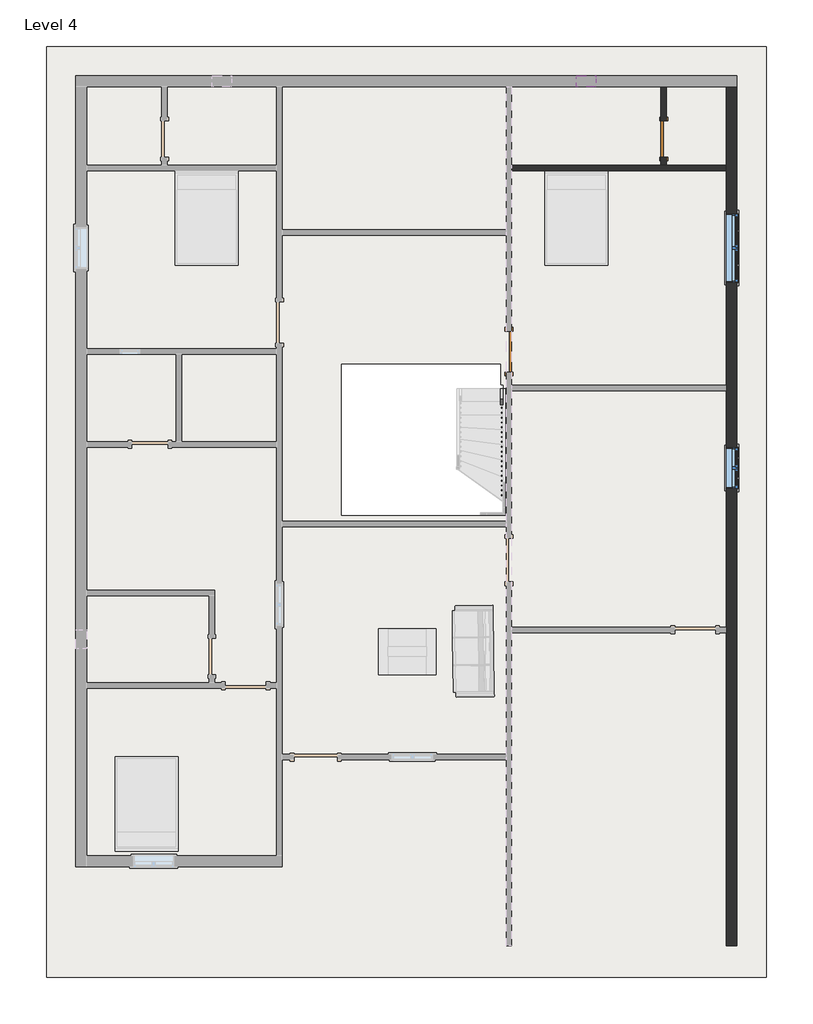
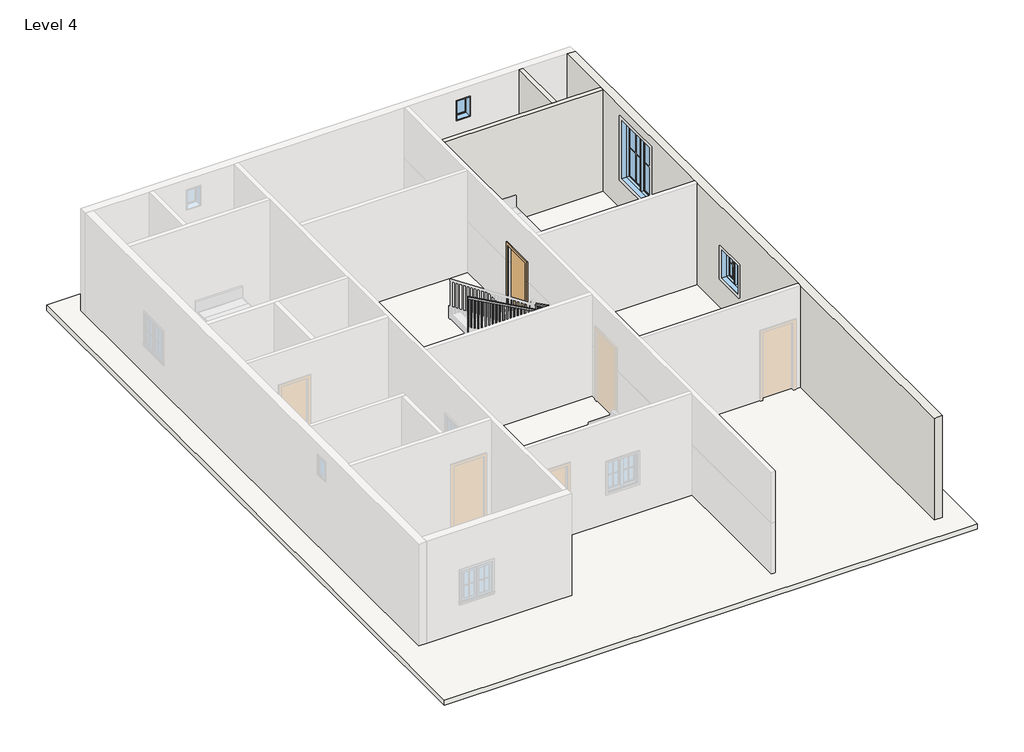
# One storey, part 2 of 3: 3 walls, 3 windows, 2 doors, 1 railing, 1 roof.
"""IFC4 building model written with IfcOpenShell, lengths in millimetres."""

from ifc_helpers import new_model, si_unit, frame, origin, place, context, project, spatial, polyline, outline, extrude, faceted_brep, transform, mapped, element, save
from components import door_f2b275c1, door_c29894e6, window_aa618e30, window_339605e1, window_9ac97e1a

model = new_model("IFC4")

# Units and contexts
model_context = context("Model", 3, world=origin())
ifc_project = project(units=[si_unit("LENGTHUNIT", "METRE", prefix="MILLI")], contexts=[model_context])

# Site, building, storey
site = spatial("IfcSite", under=ifc_project)
building = spatial("IfcBuilding", under=site)
storey = spatial("IfcBuildingStorey", under=building, Name="Level 4", Elevation=6400.8)

# Doors
placement = place(None, origin())
door_shape = door_f2b275c1(model_context)
element("IfcDoor", 1, ObjectType="Single-Flush : 30\" x 80\"", at=placement, inside=storey, context=model_context, shape_type="MappedRepresentation", body=[
    mapped(door_shape, transform((4827.3366507, 9100.7522623, 6400.8), x_axis=(0.0, -1.0, 0.0), y_axis=(1.0, 0.0, 0.0), z_axis=(0.0, 0.0, 1.0))),
])
door_2_shape = door_c29894e6(model_context)
element("IfcDoor", 2, ObjectType="Single-Flush : 34\" x 80\"", at=placement, inside=storey, context=model_context, shape_type="MappedRepresentation", body=[
    mapped(door_2_shape, transform((1583.2084916, 4643.0522623, 6400.8), x_axis=(0.0, -1.0, 0.0), y_axis=(1.0, 0.0, 0.0), z_axis=(0.0, 0.0, 1.0))),
])

# Railing
element("IfcRailing", 3, ObjectType="Handrail - Rectangular", at=placement, inside=storey, context=model_context, shape_type="SolidModel", body=[
    faceted_brep([(1456.2084916, 3870.4222402, 7484.5333333), (1456.2084916, 3870.4222402, 7427.5391458), (1405.4084916, 3870.4222402, 7427.5391458), (1405.4084916, 3870.4222402, 7484.5333333), (1456.2084916, 1506.6647172, 8686.878212), (1456.2084916, 1494.487215, 8636.078212), (1405.4084916, 1494.487215, 8636.078212), (1405.4084916, 1506.6647172, 8686.878212), (1456.2084916, 1268.9652728, 8686.878212), (1456.2084916, 1268.9652728, 8636.078212), (1405.4084916, 1319.7652728, 8636.078212), (1405.4084916, 1319.7652728, 8686.878212), (1234.4478889, 1268.9652728, 8686.878212), (1221.4006723, 1268.9652728, 8636.078212), (1221.4006723, 1319.7652728, 8636.078212), (1234.4478889, 1319.7652728, 8686.878212), (-1813.7050583, 1268.9652728, 10363.2), (-1813.7050583, 1319.7652728, 10363.2), (-1813.7050583, 1319.7652728, 10305.2247257), (-1813.7050583, 1268.9652728, 10305.2247257)], [[[0, 1, 2, 3]], [[1, 0, 4, 5]], [[2, 1, 5, 6]], [[3, 2, 6, 7]], [[0, 3, 7, 4]], [[5, 4, 8, 9]], [[6, 5, 9, 10]], [[7, 6, 10, 11]], [[4, 7, 11, 8]], [[9, 8, 12, 13]], [[10, 9, 13, 14]], [[11, 10, 14, 15]], [[8, 11, 15, 12]], [[16, 17, 18, 19]], [[13, 12, 16, 19]], [[14, 13, 19, 18]], [[15, 14, 18, 17]], [[12, 15, 17, 16]]]),
    extrude(outline(polyline([(10258.2655707, -1728.3165084), (9279.4666667, -1728.3165084), (9279.4666667, -1709.2665084), (10247.7890853, -1709.2665084), (10258.2655707, -1728.3165084)])), frame((0.0, 1284.8402728, 0.0), z_axis=(0.0, 1.0, 0.0), x_axis=(0.0, 0.0, 1.0)), (0.0, 0.0, 1.0), 19.05),
    extrude(outline(polyline([(10202.3909816, -1626.7165084), (9279.4666667, -1626.7165084), (9279.4666667, -1607.6665084), (10191.9144961, -1607.6665084), (10202.3909816, -1626.7165084)])), frame((0.0, 1284.8402728, 0.0), z_axis=(0.0, 1.0, 0.0), x_axis=(0.0, 0.0, 1.0)), (0.0, 0.0, 1.0), 19.05),
    extrude(outline(polyline([(10146.5163924, -1525.1165084), (9110.1333333, -1525.1165084), (9110.1333333, -1506.0665084), (10136.0399069, -1506.0665084), (10146.5163924, -1525.1165084)])), frame((0.0, 1284.8402728, 0.0), z_axis=(0.0, 1.0, 0.0), x_axis=(0.0, 0.0, 1.0)), (0.0, 0.0, 1.0), 19.05),
    extrude(outline(polyline([(10090.6418032, -1423.5165084), (9110.1333333, -1423.5165084), (9110.1333333, -1404.4665084), (10080.1653177, -1404.4665084), (10090.6418032, -1423.5165084)])), frame((0.0, 1284.8402728, 0.0), z_axis=(0.0, 1.0, 0.0), x_axis=(0.0, 0.0, 1.0)), (0.0, 0.0, 1.0), 19.05),
    extrude(outline(polyline([(10034.767214, -1321.9165084), (9110.1333333, -1321.9165084), (9110.1333333, -1302.8665084), (10024.2907286, -1302.8665084), (10034.767214, -1321.9165084)])), frame((0.0, 1284.8402728, 0.0), z_axis=(0.0, 1.0, 0.0), x_axis=(0.0, 0.0, 1.0)), (0.0, 0.0, 1.0), 19.05),
    extrude(outline(polyline([(9978.8926249, -1220.3165084), (8940.8, -1220.3165084), (8940.8, -1201.2665084), (9968.4161394, -1201.2665084), (9978.8926249, -1220.3165084)])), frame((0.0, 1284.8402728, 0.0), z_axis=(0.0, 1.0, 0.0), x_axis=(0.0, 0.0, 1.0)), (0.0, 0.0, 1.0), 19.05),
    extrude(outline(polyline([(9923.0180357, -1118.7165084), (8940.8, -1118.7165084), (8940.8, -1099.6665084), (9912.5415502, -1099.6665084), (9923.0180357, -1118.7165084)])), frame((0.0, 1284.8402728, 0.0), z_axis=(0.0, 1.0, 0.0), x_axis=(0.0, 0.0, 1.0)), (0.0, 0.0, 1.0), 19.05),
    extrude(outline(polyline([(9867.1434465, -1017.1165084), (8940.8, -1017.1165084), (8940.8, -998.0665084), (9856.666961, -998.0665084), (9867.1434465, -1017.1165084)])), frame((0.0, 1284.8402728, 0.0), z_axis=(0.0, 1.0, 0.0), x_axis=(0.0, 0.0, 1.0)), (0.0, 0.0, 1.0), 19.05),
    extrude(outline(polyline([(9811.2688573, -915.5165084), (8771.4666667, -915.5165084), (8771.4666667, -896.4665084), (9800.7923719, -896.4665084), (9811.2688573, -915.5165084)])), frame((0.0, 1284.8402728, 0.0), z_axis=(0.0, 1.0, 0.0), x_axis=(0.0, 0.0, 1.0)), (0.0, 0.0, 1.0), 19.05),
    extrude(outline(polyline([(9755.3942682, -813.9165084), (8771.4666667, -813.9165084), (8771.4666667, -794.8665084), (9744.9177827, -794.8665084), (9755.3942682, -813.9165084)])), frame((0.0, 1284.8402728, 0.0), z_axis=(0.0, 1.0, 0.0), x_axis=(0.0, 0.0, 1.0)), (0.0, 0.0, 1.0), 19.05),
    extrude(outline(polyline([(9699.519679, -712.3165084), (8771.4666667, -712.3165084), (8771.4666667, -693.2665084), (9689.0431935, -693.2665084), (9699.519679, -712.3165084)])), frame((0.0, 1284.8402728, 0.0), z_axis=(0.0, 1.0, 0.0), x_axis=(0.0, 0.0, 1.0)), (0.0, 0.0, 1.0), 19.05),
    extrude(outline(polyline([(9643.6450898, -610.7165084), (8602.1333333, -610.7165084), (8602.1333333, -591.6665084), (9633.1686044, -591.6665084), (9643.6450898, -610.7165084)])), frame((0.0, 1284.8402728, 0.0), z_axis=(0.0, 1.0, 0.0), x_axis=(0.0, 0.0, 1.0)), (0.0, 0.0, 1.0), 19.05),
    extrude(outline(polyline([(9587.7705007, -509.1165084), (8602.1333333, -509.1165084), (8602.1333333, -490.0665084), (9577.2940152, -490.0665084), (9587.7705007, -509.1165084)])), frame((0.0, 1284.8402728, 0.0), z_axis=(0.0, 1.0, 0.0), x_axis=(0.0, 0.0, 1.0)), (0.0, 0.0, 1.0), 19.05),
    extrude(outline(polyline([(9531.8959115, -407.5165084), (8602.1333333, -407.5165084), (8602.1333333, -388.4665084), (9521.419426, -388.4665084), (9531.8959115, -407.5165084)])), frame((0.0, 1284.8402728, 0.0), z_axis=(0.0, 1.0, 0.0), x_axis=(0.0, 0.0, 1.0)), (0.0, 0.0, 1.0), 19.05),
    extrude(outline(polyline([(9476.0213223, -305.9165084), (8432.8, -305.9165084), (8432.8, -286.8665084), (9465.5448368, -286.8665084), (9476.0213223, -305.9165084)])), frame((0.0, 1284.8402728, 0.0), z_axis=(0.0, 1.0, 0.0), x_axis=(0.0, 0.0, 1.0)), (0.0, 0.0, 1.0), 19.05),
    extrude(outline(polyline([(9420.1467331, -204.3165084), (8432.8, -204.3165084), (8432.8, -185.2665084), (9409.6702477, -185.2665084), (9420.1467331, -204.3165084)])), frame((0.0, 1284.8402728, 0.0), z_axis=(0.0, 1.0, 0.0), x_axis=(0.0, 0.0, 1.0)), (0.0, 0.0, 1.0), 19.05),
    extrude(outline(polyline([(9364.272144, -102.7165084), (8432.8, -102.7165084), (8432.8, -83.6665084), (9353.7956585, -83.6665084), (9364.272144, -102.7165084)])), frame((0.0, 1284.8402728, 0.0), z_axis=(0.0, 1.0, 0.0), x_axis=(0.0, 0.0, 1.0)), (0.0, 0.0, 1.0), 19.05),
    extrude(outline(polyline([(9308.3975548, -1.1165084), (8263.4666667, -1.1165084), (8263.4666667, 17.9334916), (9297.9210693, 17.9334916), (9308.3975548, -1.1165084)])), frame((0.0, 1284.8402728, 0.0), z_axis=(0.0, 1.0, 0.0), x_axis=(0.0, 0.0, 1.0)), (0.0, 0.0, 1.0), 19.05),
    extrude(outline(polyline([(9252.5229656, 100.4834916), (8263.4666667, 100.4834916), (8263.4666667, 119.5334916), (9242.0464801, 119.5334916), (9252.5229656, 100.4834916)])), frame((0.0, 1284.8402728, 0.0), z_axis=(0.0, 1.0, 0.0), x_axis=(0.0, 0.0, 1.0)), (0.0, 0.0, 1.0), 19.05),
    extrude(outline(polyline([(9196.6483764, 202.0834916), (8263.4666667, 202.0834916), (8263.4666667, 221.1334916), (9186.171891, 221.1334916), (9196.6483764, 202.0834916)])), frame((0.0, 1284.8402728, 0.0), z_axis=(0.0, 1.0, 0.0), x_axis=(0.0, 0.0, 1.0)), (0.0, 0.0, 1.0), 19.05),
    extrude(outline(polyline([(9140.7737873, 303.6834916), (8094.1333333, 303.6834916), (8094.1333333, 322.7334916), (9130.2973018, 322.7334916), (9140.7737873, 303.6834916)])), frame((0.0, 1284.8402728, 0.0), z_axis=(0.0, 1.0, 0.0), x_axis=(0.0, 0.0, 1.0)), (0.0, 0.0, 1.0), 19.05),
    extrude(outline(polyline([(9084.8991981, 405.2834916), (8094.1333333, 405.2834916), (8094.1333333, 424.3334916), (9074.4227126, 424.3334916), (9084.8991981, 405.2834916)])), frame((0.0, 1284.8402728, 0.0), z_axis=(0.0, 1.0, 0.0), x_axis=(0.0, 0.0, 1.0)), (0.0, 0.0, 1.0), 19.05),
    extrude(outline(polyline([(9029.0246089, 506.8834916), (8094.1333333, 506.8834916), (8094.1333333, 525.9334916), (9018.5481235, 525.9334916), (9029.0246089, 506.8834916)])), frame((0.0, 1284.8402728, 0.0), z_axis=(0.0, 1.0, 0.0), x_axis=(0.0, 0.0, 1.0)), (0.0, 0.0, 1.0), 19.05),
    extrude(outline(polyline([(8973.1500198, 608.4834916), (7924.8, 608.4834916), (7924.8, 627.5334916), (8962.6735343, 627.5334916), (8973.1500198, 608.4834916)])), frame((0.0, 1284.8402728, 0.0), z_axis=(0.0, 1.0, 0.0), x_axis=(0.0, 0.0, 1.0)), (0.0, 0.0, 1.0), 19.05),
    extrude(outline(polyline([(8917.2754306, 710.0834916), (7924.8, 710.0834916), (7924.8, 729.1334916), (8906.7989451, 729.1334916), (8917.2754306, 710.0834916)])), frame((0.0, 1284.8402728, 0.0), z_axis=(0.0, 1.0, 0.0), x_axis=(0.0, 0.0, 1.0)), (0.0, 0.0, 1.0), 19.05),
    extrude(outline(polyline([(8861.4008414, 811.6834916), (7924.8, 811.6834916), (7924.8, 830.7334916), (8850.9243559, 830.7334916), (8861.4008414, 811.6834916)])), frame((0.0, 1284.8402728, 0.0), z_axis=(0.0, 1.0, 0.0), x_axis=(0.0, 0.0, 1.0)), (0.0, 0.0, 1.0), 19.05),
    extrude(outline(polyline([(8805.5262522, 913.2834916), (7924.8, 913.2834916), (7924.8, 932.3334916), (8795.0497668, 932.3334916), (8805.5262522, 913.2834916)])), frame((0.0, 1284.8402728, 0.0), z_axis=(0.0, 1.0, 0.0), x_axis=(0.0, 0.0, 1.0)), (0.0, 0.0, 1.0), 19.05),
    extrude(outline(polyline([(8749.6516631, 1014.8834916), (7755.4666667, 1014.8834916), (7755.4666667, 1033.9334916), (8739.1751776, 1033.9334916), (8749.6516631, 1014.8834916)])), frame((0.0, 1284.8402728, 0.0), z_axis=(0.0, 1.0, 0.0), x_axis=(0.0, 0.0, 1.0)), (0.0, 0.0, 1.0), 19.05),
    extrude(outline(polyline([(8693.7770739, 1116.4834916), (7755.4666667, 1116.4834916), (7755.4666667, 1135.5334916), (8683.3005884, 1135.5334916), (8693.7770739, 1116.4834916)])), frame((0.0, 1284.8402728, 0.0), z_axis=(0.0, 1.0, 0.0), x_axis=(0.0, 0.0, 1.0)), (0.0, 0.0, 1.0), 19.05),
    extrude(outline(polyline([(8637.9024847, 1218.0834916), (7755.4666667, 1218.0834916), (7755.4666667, 1237.1334916), (8627.4259992, 1237.1334916), (8637.9024847, 1218.0834916)])), frame((0.0, 1284.8402728, 0.0), z_axis=(0.0, 1.0, 0.0), x_axis=(0.0, 0.0, 1.0)), (0.0, 0.0, 1.0), 19.05),
    extrude(outline(polyline([(1338.7334916, 1284.8402728), (1319.6834916, 1284.8402728), (1319.6834916, 1303.8902728), (1338.7334916, 1303.8902728), (1338.7334916, 1284.8402728)])), frame((0.0, 0.0, 7755.4666667), z_axis=(0.0, 0.0, 1.0), x_axis=(1.0, 0.0, 0.0)), (0.0, 0.0, 1.0), 880.6115453),
    extrude(outline(polyline([(1440.3334916, 1339.9472402), (1440.3334916, 1320.8972402), (1421.2834916, 1320.8972402), (1421.2834916, 1339.9472402), (1440.3334916, 1339.9472402)])), frame((0.0, 0.0, 7755.4666667), z_axis=(0.0, 0.0, 1.0), x_axis=(1.0, 0.0, 0.0)), (0.0, 0.0, 1.0), 880.6115453),
    extrude(outline(polyline([(1440.3334916, 1441.5472402), (1440.3334916, 1422.4972402), (1421.2834916, 1422.4972402), (1421.2834916, 1441.5472402), (1440.3334916, 1441.5472402)])), frame((0.0, 0.0, 7755.4666667), z_axis=(0.0, 0.0, 1.0), x_axis=(1.0, 0.0, 0.0)), (0.0, 0.0, 1.0), 880.6115453),
    extrude(outline(polyline([(1543.1472402, 8611.3268864), (1543.1472402, 7755.4666667), (1524.0972402, 7755.4666667), (1524.0972402, 8621.016827), (1543.1472402, 8611.3268864)])), frame((1421.2834916, 0.0, 0.0), z_axis=(1.0, 0.0, 0.0), x_axis=(0.0, 1.0, 0.0)), (0.0, 0.0, 1.0), 19.05),
    extrude(outline(polyline([(1644.7472402, 8559.6472033), (1644.7472402, 7586.1333333), (1625.6972402, 7586.1333333), (1625.6972402, 8569.3371439), (1644.7472402, 8559.6472033)])), frame((1421.2834916, 0.0, 0.0), z_axis=(1.0, 0.0, 0.0), x_axis=(0.0, 1.0, 0.0)), (0.0, 0.0, 1.0), 19.05),
    extrude(outline(polyline([(1746.3472402, 8507.9675203), (1746.3472402, 7586.1333333), (1727.2972402, 7586.1333333), (1727.2972402, 8517.6574608), (1746.3472402, 8507.9675203)])), frame((1421.2834916, 0.0, 0.0), z_axis=(1.0, 0.0, 0.0), x_axis=(0.0, 1.0, 0.0)), (0.0, 0.0, 1.0), 19.05),
    extrude(outline(polyline([(1847.9472402, 8456.2878372), (1847.9472402, 7586.1333333), (1828.8972402, 7586.1333333), (1828.8972402, 8465.9777778), (1847.9472402, 8456.2878372)])), frame((1421.2834916, 0.0, 0.0), z_axis=(1.0, 0.0, 0.0), x_axis=(0.0, 1.0, 0.0)), (0.0, 0.0, 1.0), 19.05),
    extrude(outline(polyline([(1949.5472402, 8404.6081541), (1949.5472402, 7586.1333333), (1930.4972402, 7586.1333333), (1930.4972402, 8414.2980947), (1949.5472402, 8404.6081541)])), frame((1421.2834916, 0.0, 0.0), z_axis=(1.0, 0.0, 0.0), x_axis=(0.0, 1.0, 0.0)), (0.0, 0.0, 1.0), 19.05),
    extrude(outline(polyline([(2051.1472402, 8352.928471), (2051.1472402, 7416.8), (2032.0972402, 7416.8), (2032.0972402, 8362.6184116), (2051.1472402, 8352.928471)])), frame((1421.2834916, 0.0, 0.0), z_axis=(1.0, 0.0, 0.0), x_axis=(0.0, 1.0, 0.0)), (0.0, 0.0, 1.0), 19.05),
    extrude(outline(polyline([(2152.7472402, 8301.2487879), (2152.7472402, 7416.8), (2133.6972402, 7416.8), (2133.6972402, 8310.9387285), (2152.7472402, 8301.2487879)])), frame((1421.2834916, 0.0, 0.0), z_axis=(1.0, 0.0, 0.0), x_axis=(0.0, 1.0, 0.0)), (0.0, 0.0, 1.0), 19.05),
    extrude(outline(polyline([(2254.3472402, 8249.5691048), (2254.3472402, 7416.8), (2235.2972402, 7416.8), (2235.2972402, 8259.2590454), (2254.3472402, 8249.5691048)])), frame((1421.2834916, 0.0, 0.0), z_axis=(1.0, 0.0, 0.0), x_axis=(0.0, 1.0, 0.0)), (0.0, 0.0, 1.0), 19.05),
    extrude(outline(polyline([(2355.9472402, 8197.8894218), (2355.9472402, 7416.8), (2336.8972402, 7416.8), (2336.8972402, 8207.5793623), (2355.9472402, 8197.8894218)])), frame((1421.2834916, 0.0, 0.0), z_axis=(1.0, 0.0, 0.0), x_axis=(0.0, 1.0, 0.0)), (0.0, 0.0, 1.0), 19.05),
    extrude(outline(polyline([(2457.5472402, 8146.2097387), (2457.5472402, 7247.4666667), (2438.4972402, 7247.4666667), (2438.4972402, 8155.8996793), (2457.5472402, 8146.2097387)])), frame((1421.2834916, 0.0, 0.0), z_axis=(1.0, 0.0, 0.0), x_axis=(0.0, 1.0, 0.0)), (0.0, 0.0, 1.0), 19.05),
    extrude(outline(polyline([(2559.1472402, 8094.5300556), (2559.1472402, 7247.4666667), (2540.0972402, 7247.4666667), (2540.0972402, 8104.2199962), (2559.1472402, 8094.5300556)])), frame((1421.2834916, 0.0, 0.0), z_axis=(1.0, 0.0, 0.0), x_axis=(0.0, 1.0, 0.0)), (0.0, 0.0, 1.0), 19.05),
    extrude(outline(polyline([(2660.7472402, 8042.8503725), (2660.7472402, 7247.4666667), (2641.6972402, 7247.4666667), (2641.6972402, 8052.5403131), (2660.7472402, 8042.8503725)])), frame((1421.2834916, 0.0, 0.0), z_axis=(1.0, 0.0, 0.0), x_axis=(0.0, 1.0, 0.0)), (0.0, 0.0, 1.0), 19.05),
    extrude(outline(polyline([(2762.3472402, 7991.1706894), (2762.3472402, 7078.1333333), (2743.2972402, 7078.1333333), (2743.2972402, 8000.86063), (2762.3472402, 7991.1706894)])), frame((1421.2834916, 0.0, 0.0), z_axis=(1.0, 0.0, 0.0), x_axis=(0.0, 1.0, 0.0)), (0.0, 0.0, 1.0), 19.05),
    extrude(outline(polyline([(2863.9472402, 7939.4910064), (2863.9472402, 7078.1333333), (2844.8972402, 7078.1333333), (2844.8972402, 7949.1809469), (2863.9472402, 7939.4910064)])), frame((1421.2834916, 0.0, 0.0), z_axis=(1.0, 0.0, 0.0), x_axis=(0.0, 1.0, 0.0)), (0.0, 0.0, 1.0), 19.05),
    extrude(outline(polyline([(2965.5472402, 7887.8113233), (2965.5472402, 7078.1333333), (2946.4972402, 7078.1333333), (2946.4972402, 7897.5012638), (2965.5472402, 7887.8113233)])), frame((1421.2834916, 0.0, 0.0), z_axis=(1.0, 0.0, 0.0), x_axis=(0.0, 1.0, 0.0)), (0.0, 0.0, 1.0), 19.05),
    extrude(outline(polyline([(3067.1472402, 7836.1316402), (3067.1472402, 6908.8), (3048.0972402, 6908.8), (3048.0972402, 7845.8215808), (3067.1472402, 7836.1316402)])), frame((1421.2834916, 0.0, 0.0), z_axis=(1.0, 0.0, 0.0), x_axis=(0.0, 1.0, 0.0)), (0.0, 0.0, 1.0), 19.05),
    extrude(outline(polyline([(3168.7472402, 7784.4519571), (3168.7472402, 6908.8), (3149.6972402, 6908.8), (3149.6972402, 7794.1418977), (3168.7472402, 7784.4519571)])), frame((1421.2834916, 0.0, 0.0), z_axis=(1.0, 0.0, 0.0), x_axis=(0.0, 1.0, 0.0)), (0.0, 0.0, 1.0), 19.05),
    extrude(outline(polyline([(3270.3472402, 7732.772274), (3270.3472402, 6908.8), (3251.2972402, 6908.8), (3251.2972402, 7742.4622146), (3270.3472402, 7732.772274)])), frame((1421.2834916, 0.0, 0.0), z_axis=(1.0, 0.0, 0.0), x_axis=(0.0, 1.0, 0.0)), (0.0, 0.0, 1.0), 19.05),
    extrude(outline(polyline([(3371.9472402, 7681.0925909), (3371.9472402, 6739.4666667), (3352.8972402, 6739.4666667), (3352.8972402, 7690.7825315), (3371.9472402, 7681.0925909)])), frame((1421.2834916, 0.0, 0.0), z_axis=(1.0, 0.0, 0.0), x_axis=(0.0, 1.0, 0.0)), (0.0, 0.0, 1.0), 19.05),
    extrude(outline(polyline([(3473.5472402, 7629.4129079), (3473.5472402, 6739.4666667), (3454.4972402, 6739.4666667), (3454.4972402, 7639.1028484), (3473.5472402, 7629.4129079)])), frame((1421.2834916, 0.0, 0.0), z_axis=(1.0, 0.0, 0.0), x_axis=(0.0, 1.0, 0.0)), (0.0, 0.0, 1.0), 19.05),
    extrude(outline(polyline([(3575.1472402, 7577.7332248), (3575.1472402, 6739.4666667), (3556.0972402, 6739.4666667), (3556.0972402, 7587.4231654), (3575.1472402, 7577.7332248)])), frame((1421.2834916, 0.0, 0.0), z_axis=(1.0, 0.0, 0.0), x_axis=(0.0, 1.0, 0.0)), (0.0, 0.0, 1.0), 19.05),
    extrude(outline(polyline([(3676.7472402, 7526.0535417), (3676.7472402, 6570.1333333), (3657.6972402, 6570.1333333), (3657.6972402, 7535.7434823), (3676.7472402, 7526.0535417)])), frame((1421.2834916, 0.0, 0.0), z_axis=(1.0, 0.0, 0.0), x_axis=(0.0, 1.0, 0.0)), (0.0, 0.0, 1.0), 19.05),
    extrude(outline(polyline([(3778.3472402, 7474.3738586), (3778.3472402, 6570.1333333), (3759.2972402, 6570.1333333), (3759.2972402, 7484.0637992), (3778.3472402, 7474.3738586)])), frame((1421.2834916, 0.0, 0.0), z_axis=(1.0, 0.0, 0.0), x_axis=(0.0, 1.0, 0.0)), (0.0, 0.0, 1.0), 19.05),
    extrude(outline(polyline([(1440.3334916, 1303.8902728), (1440.3334916, 1284.8402728), (1421.2834916, 1284.8402728), (1421.2834916, 1303.8902728), (1440.3334916, 1303.8902728)])), frame((0.0, 0.0, 7755.4666667), z_axis=(0.0, 0.0, 1.0), x_axis=(1.0, 0.0, 0.0)), (0.0, 0.0, 1.0), 880.6115453),
    extrude(outline(polyline([(10305.2247257, -1813.7050583), (9279.4666667, -1813.7050583), (9279.4666667, -1794.6550583), (10294.7482402, -1794.6550583), (10305.2247257, -1813.7050583)])), frame((0.0, 1284.8402728, 0.0), z_axis=(0.0, 1.0, 0.0), x_axis=(0.0, 0.0, 1.0)), (0.0, 0.0, 1.0), 19.05),
    extrude(outline(polyline([(3870.4222402, 7427.5391458), (3870.4222402, 6570.1333333), (3851.3722402, 6570.1333333), (3851.3722402, 7437.2290864), (3870.4222402, 7427.5391458)])), frame((1421.2834916, 0.0, 0.0), z_axis=(1.0, 0.0, 0.0), x_axis=(0.0, 1.0, 0.0)), (0.0, 0.0, 1.0), 19.05),
])

# Roof
element("IfcRoof", 4, ObjectType="Generic - 12\"", at=placement, inside=storey, context=model_context, shape_type="SweptSolid", body=[
    extrude(outline(polyline([(-8113.2415084, -8469.6977377), (-8113.2415084, 11037.5022623), (6974.3584916, 11037.5022623), (6974.3584916, -8469.6977377), (-8113.2415084, -8469.6977377)]), holes=[polyline([(1404.6885894, 4375.6877175), (-1922.9455737, 4375.6877175), (-1922.9455737, 1218.1652728), (1404.6885894, 1218.1652728), (1404.6885894, 1268.9652728), (1456.2084916, 1268.9652728), (1456.2084916, 3938.2022623), (1404.6885894, 3938.2022623), (1404.6885894, 4375.6877175)])]), frame((0.0, 0.0, 6248.4), z_axis=(0.0, 0.0, 1.0), x_axis=(1.0, 0.0, 0.0)), (0.0, 0.0, 1.0), 152.4),
])

# Walls
element("IfcWall", 5, ObjectType="9\"", at=placement, inside=storey, context=model_context, shape_type="Brep", body=[
    faceted_brep([(6136.1584916, 10199.3022623, 6400.8), (6136.1584916, 8548.3022623, 6400.8), (6136.1584916, 8434.0022623, 6400.8), (6136.1584916, 3938.2022623, 6400.8), (6136.1584916, 3823.9022623, 6400.8), (6136.1584916, -1129.0977377, 6400.8), (6136.1584916, -1243.3977377, 6400.8), (6136.1584916, -7802.9477377, 6400.8), (6136.1584916, -7802.9477377, 9448.8), (6136.1584916, -1243.3977377, 9448.8), (6136.1584916, -1129.0977377, 9448.8), (6136.1584916, 3823.9022623, 9448.8), (6136.1584916, 3938.2022623, 9448.8), (6136.1584916, 8434.0022623, 9448.8), (6136.1584916, 8548.3022623, 9448.8), (6136.1584916, 10199.3022623, 9448.8), (6136.1584916, 1772.8522623, 8229.6), (6136.1584916, 1772.8522623, 7315.2), (6136.1584916, 2636.4522623, 7315.2), (6136.1584916, 2636.4522623, 8229.6), (6136.1584916, 6090.8522623, 9144.0), (6136.1584916, 6090.8522623, 7315.2), (6136.1584916, 7538.6522623, 7315.2), (6136.1584916, 7538.6522623, 9144.0), (6364.7584916, 10199.3022623, 6400.8), (6364.7584916, 10199.3022623, 9448.8), (6364.7584916, -7802.9477377, 9448.8), (6364.7584916, -7802.9477377, 6400.8), (6364.7584916, 1772.8522623, 8229.6), (6364.7584916, 2636.4522623, 8229.6), (6364.7584916, 2636.4522623, 7315.2), (6364.7584916, 1772.8522623, 7315.2), (6364.7584916, 6090.8522623, 9144.0), (6364.7584916, 7538.6522623, 9144.0), (6364.7584916, 7538.6522623, 7315.2), (6364.7584916, 6090.8522623, 7315.2)], [[[0, 1, 2, 3, 4, 5, 6, 7, 8, 9, 10, 11, 12, 13, 14, 15], [16, 17, 18, 19], [20, 21, 22, 23]], [[24, 25, 26, 27], [28, 29, 30, 31], [32, 33, 34, 35]], [[7, 6, 5, 4, 3, 2, 1, 0, 24, 27]], [[8, 7, 27, 26]], [[0, 15, 25, 24]], [[17, 16, 28, 31]], [[18, 17, 31, 30]], [[19, 18, 30, 29]], [[16, 19, 29, 28]], [[21, 20, 32, 35]], [[22, 21, 35, 34]], [[23, 22, 34, 33]], [[20, 23, 33, 32]], [[15, 14, 13, 12, 11, 10, 9, 8, 26, 25]]]),
])
element("IfcWall", 6, ObjectType="WALL4.5\"", at=placement, inside=storey, context=model_context, shape_type="SweptSolid", body=[
    extrude(outline(polyline([(8719.7522623, 8432.8), (8719.7522623, 6400.8), (8548.3022623, 6400.8), (8548.3022623, 9448.8), (10199.3022623, 9448.8), (10199.3022623, 6400.8), (9481.7522623, 6400.8), (9481.7522623, 8432.8), (8719.7522623, 8432.8)])), frame((4770.1866507, 0.0, 0.0), z_axis=(1.0, 0.0, 0.0), x_axis=(0.0, 1.0, 0.0)), (0.0, 0.0, 1.0), 114.3),
])
element("IfcWall", 7, ObjectType="WALL4.5\"", at=placement, inside=storey, context=model_context, shape_type="Brep", body=[
    faceted_brep([(1640.3584916, 8434.0022623, 9448.8), (1640.3584916, 8434.0022623, 6400.8), (6136.1584916, 8434.0022623, 6400.8), (6136.1584916, 8434.0022623, 9448.8), (1640.3584916, 8548.3022623, 6400.8), (1640.3584916, 8548.3022623, 9448.8), (4770.1866507, 8548.3022623, 9448.8), (4884.4866507, 8548.3022623, 9448.8), (6136.1584916, 8548.3022623, 9448.8), (6136.1584916, 8548.3022623, 6400.8), (4884.4866507, 8548.3022623, 6400.8), (4770.1866507, 8548.3022623, 6400.8)], [[[0, 1, 2, 3]], [[4, 5, 6, 7, 8, 9, 10, 11]], [[2, 1, 4, 11, 10, 9]], [[3, 2, 9, 8]], [[0, 3, 8, 7, 6, 5]], [[0, 5, 4, 1]]]),
])

# Windows
window_shape = window_aa618e30(model_context)
element("IfcWindow", 8, ObjectType="Fixed : 16\" x 24\"", at=placement, inside=storey, context=model_context, shape_type="MappedRepresentation", body=[
    mapped(window_shape, transform((3243.3725711, 10313.6022623, 7620.0), x_axis=(1.0, 0.0, 0.0), y_axis=(0.0, 1.0, 0.0), z_axis=(0.0, 0.0, 1.0))),
])
window_2_shape = window_339605e1(model_context)
element("IfcWindow", 9, ObjectType="Window-Casement-Double : 34\" x 36\"", at=placement, inside=storey, context=model_context, shape_type="MappedRepresentation", body=[
    mapped(window_2_shape, transform((6250.4584916, 2204.6522623, 6400.8), x_axis=(0.0, -1.0, 0.0), y_axis=(1.0, 0.0, 0.0), z_axis=(0.0, 0.0, 1.0))),
])
window_3_shape = window_9ac97e1a(model_context)
element("IfcWindow", 10, ObjectType="Window-Casement-Double : 57\" x 72\"", at=placement, inside=storey, context=model_context, shape_type="MappedRepresentation", body=[
    mapped(window_3_shape, transform((6250.4584916, 6814.7522623, 6400.8), x_axis=(0.0, -1.0, 0.0), y_axis=(1.0, 0.0, 0.0), z_axis=(0.0, 0.0, 1.0))),
])

save(model, "model.ifc")

# Revit data of these elements
# Type "Single-Flush : 30\" x 80\""
#   Type Mark = "5"
#   Construction Type Id = "MDOOR"
#   Assembly Code = "C1020"
#   Analytic Construction = "Metal"
#   Thickness = 0' - 2"
#   Heat Transfer Coefficient (U) = 0.651978 BTU/(h·ft²·°F)
#   Height = 6' - 8"
#   Trim Projection Ext = 0' - 1"
#   Trim Projection Int = 0' - 1"
#   Trim Width = 0' - 3"
#   Width = 2' - 6"
#   Define Thermal Properties by = 1
#   Define Thermal Properties by = 1
#   Door Material = Door - Panel
#   Frame Material = Door - Frame
#   Visual Light Transmittance = 0
#   Solar Heat Gain Coefficient = 0
#   Function = (empty or 0)
#   Wall Closure = (empty or 0)
# Type "Single-Flush : 34\" x 80\""
#   Type Mark = "7"
#   Construction Type Id = "MDOOR"
#   Assembly Code = "C1020"
#   Analytic Construction = "Metal"
#   Thickness = 0' - 2"
#   Heat Transfer Coefficient (U) = 0.651978 BTU/(h·ft²·°F)
#   Height = 6' - 8"
#   Trim Projection Ext = 0' - 1"
#   Trim Projection Int = 0' - 1"
#   Trim Width = 0' - 3"
#   Width = 2' - 10"
#   Define Thermal Properties by = 1
#   Define Thermal Properties by = 1
#   Door Material = Door - Panel
#   Frame Material = Door - Frame
#   Visual Light Transmittance = 0
#   Solar Heat Gain Coefficient = 0
#   Function = (empty or 0)
#   Wall Closure = (empty or 0)
# Type "Handrail - Rectangular"
#   Assembly Code = "C2010400"
#   built-in parameter 1008612 = 0.0416667 (stored number, unit not read)
#   built-in parameter 1008611 = 0.0416667 (stored number, unit not read)
#   built-in parameter 1008609 = 0.333333 (stored number, unit not read)
#   built-in parameter 1008604 = 0.166667 (stored number, unit not read)
#   built-in parameter 1008603 = 0.166667 (stored number, unit not read)
#   Railing Height = 3' - 0"
#   built-in parameter 1008630 = 2
#   built-in parameter 1008610 = 2
#   built-in parameter 1008618 = Baluster - Square : 3/4"
# Type "Generic - 12\""
#   Assembly Code = "B1020"
#   Layers, outside or top first: 0' - 6" no material (function 1)
# Type "9\""
#   Assembly Code = "B2010"
#   Layers, outside or top first: 0' - 9" no material (function 1)
# Type "WALL4.5\""
#   Assembly Code = "B2010"
#   Layers, outside or top first: 0' - 4 1/2" no material (function 1)
# Type "Fixed : 16\" x 24\""
#   Type Mark = "4"
#   Construction Type Id = "GSP4R"
#   Assembly Code = "B2020100"
#   Analytic Construction = "1/8 in Pilkington single glazing"
#   Visual Light Transmittance = 0.9
#   Solar Heat Gain Coefficient = 0.78
#   Heat Transfer Coefficient (U) = 0.6496 BTU/(h·ft²·°F)
#   Height = 2' - 0"
#   Default Sill Height = 3' - 0"
#   Width = 1' - 4"
#   Window Inset = 0' - 0 3/4"
#   Define Thermal Properties by = 1
#   Define Thermal Properties by = 1
#   Glass Pane Material = Glass
#   Sash Material = Sash
#   Wall Closure = (empty or 0)
# Type "Window-Casement-Double : 34\" x 36\""
#   Type Mark = "14"
#   Fire Rating = "0.5h"
#   Assembly Code = "B2020100"
#   Analytic Construction = "Double glazing - domestic"
#   Frame Extension [instance default] = 0' - 0 1/4"
#   Window Inset [instance default] = 0' - 0"
#   Wall Thickness [instance default] = 0' - 6"
#   Interior Wall Closure [instance default] = 0' - 2 1/4"
#   Half Width = 1' - 5"
#   Visual Light Transmittance = 0.81
#   Thermal Resistance (R) = 1.8146 (h·ft²·°F)/BTU
#   Solar Heat Gain Coefficient = 0.76
#   Rough Width = 2' - 10 1/2"
#   Rough Height = 3' - 0 1/2"
#   Height = 3' - 0"
#   Heat Transfer Coefficient (U) = 0.5511 BTU/(h·ft²·°F)
#   Exterior Wall Closure [instance default] = 0' - 1 1/4"
#   Extension Jamb [instance default] = 0' - 2 1/4"
#   Default Sill Height = 3' - 0"
#   Width = 2' - 10"
#   Define Thermal Properties by = 0
#   Muntin Visibility = yes
#   Interior Trim Visibility [instance default] = yes
#   Exterior Trim Visibility [instance default] = yes
#   Extension Jamb Visibility [instance default] = yes
#   Interior Trim Material = Wood - Stained
#   Muntin Pattern = Muntin Pattern_2x2 : Muntin Pattern_2x2
#   Interior Trim = Trim-Window-Interior-Flat : Picture Frame
#   Interior Frame Material = Wood - Stained
#   Glass Panel Material = Glass
#   Exterior Trim Material = Clad - White
#   Exterior Trim = Trim-Window-Exterior-Flat : with Sill
#   Exterior Frame Material = Clad - White
#   Wall Closure = (empty or 0)
# Type "Window-Casement-Double : 57\" x 72\""
#   Type Mark = "17"
#   Fire Rating = "0.5h"
#   Assembly Code = "B2020100"
#   Analytic Construction = "Double glazing - domestic"
#   Frame Extension [instance default] = 0' - 0 1/4"
#   Window Inset [instance default] = 0' - 0"
#   Wall Thickness [instance default] = 0' - 6"
#   Interior Wall Closure [instance default] = 0' - 2 1/4"
#   Half Width = 2' - 4 1/2"
#   Visual Light Transmittance = 0.81
#   Thermal Resistance (R) = 1.8146 (h·ft²·°F)/BTU
#   Solar Heat Gain Coefficient = 0.76
#   Rough Width = 4' - 9 1/2"
#   Rough Height = 6' - 0 1/2"
#   Height = 6' - 0"
#   Heat Transfer Coefficient (U) = 0.5511 BTU/(h·ft²·°F)
#   Exterior Wall Closure [instance default] = 0' - 1 1/4"
#   Extension Jamb [instance default] = 0' - 2 1/4"
#   Default Sill Height = 3' - 0"
#   Width = 4' - 9"
#   Define Thermal Properties by = 0
#   Muntin Visibility = yes
#   Interior Trim Visibility [instance default] = yes
#   Exterior Trim Visibility [instance default] = yes
#   Extension Jamb Visibility [instance default] = yes
#   Interior Trim Material = Wood - Stained
#   Muntin Pattern = Muntin Pattern_2x2 : Muntin Pattern_2x2
#   Interior Trim = Trim-Window-Interior-Flat : Picture Frame
#   Interior Frame Material = Wood - Stained
#   Glass Panel Material = Glass
#   Exterior Trim Material = Clad - White
#   Exterior Trim = Trim-Window-Exterior-Flat : with Sill
#   Exterior Frame Material = Clad - White
#   Wall Closure = (empty or 0)
# Element 1 (IfcDoor, "Single-Flush : 30\" x 80\"")
#   Phase Created = New Construction
#   Materials on its faces: "Door - Frame", "Door - Panel"
# Element 2 (IfcDoor, "Single-Flush : 34\" x 80\"")
#   Phase Created = New Construction
#   Materials on its faces: "Door - Frame", "Door - Panel"
# Element 3 (IfcRailing, "Handrail - Rectangular")
#   Phase Created = New Construction
# Element 4 (IfcRoof, "Generic - 12\"")
#   built-in parameter 1001705 = 21 (stored number, unit not read)
#   built-in parameter 1001701 = -0.5 (stored number, unit not read)
#   built-in parameter 1001710 = 33615
#   Phase Created = New Construction
#   Materials on its faces: "Default Roof", "legs", "Tile, Mosaic, Gray"
# Element 5 (IfcWall, "9\"")
#   Top Offset = 0' - 0"
#   Base Offset = 0' - 0"
#   Unconnected Height = 10' - 0"
#   wall height = 10' - 0"
#   Phase Created = New Construction
#   Base Constraint = Level 4
#   Materials on its faces: "Default Wall", "legs"
# Elements 6, 7 (IfcWall, "WALL4.5\"")
#   Top Offset = 0' - 0"
#   Base Offset = 0' - 0"
#   Unconnected Height = 10' - 0"
#   wall height = 10' - 0"
#   Phase Created = New Construction
#   Base Constraint = Level 4
#   Materials on its faces: "Default Wall"
# Element 8 (IfcWindow, "Fixed : 16\" x 24\"")
#   Mark = "22"
#   Phase Created = New Construction
#   Materials on its faces: "Sash", "Glass"
# Element 9 (IfcWindow, "Window-Casement-Double : 34\" x 36\"")
#   Mark = "28"
#   Window Inset = 0' - 0"
#   Interior Wall Closure = 0' - 2 1/4"
#   Frame Extension = 0' - 0 1/4"
#   Exterior Wall Closure = 0' - 1 1/4"
#   Interior Trim Visibility = yes
#   Exterior Trim Visibility = yes
#   Phase Created = New Construction
#   Materials on its faces: "Wood - Stained", "Glass", "Clad - White"
# Element 10 (IfcWindow, "Window-Casement-Double : 57\" x 72\"")
#   Mark = "29"
#   Window Inset = 0' - 0"
#   Interior Wall Closure = 0' - 2 1/4"
#   Frame Extension = 0' - 0 1/4"
#   Exterior Wall Closure = 0' - 1 1/4"
#   Interior Trim Visibility = yes
#   Exterior Trim Visibility = yes
#   Phase Created = New Construction
#   Materials on its faces: "Wood - Stained", "Glass", "Clad - White"
# Materials
#   "Door - Panel": class "Wood", colour RGB 210 159 95, transparency 0, Cost = 0
#   "Door - Frame": colour RGB 118 70 51, transparency 0, Cost = 0
#   "Glass": class "Glass", colour RGB 0 128 192, transparency 0.75, Description = "Soda Lime Glass", Cost = 0
#   "Sash": class "Wood", colour RGB 224 178 126, transparency 0, Cost = 0
#   "Wood - Stained": class "Wood", colour RGB 224 178 126, transparency 0, Cost = 0
#   "Clad - White": class "Wood", colour RGB 242 242 238, transparency 0, Cost = 0
#   "Default Roof": colour RGB 88 101 114, transparency 0, Cost = 0
#   "legs": colour RGB 90 73 37, transparency 0, Cost = 0
#   "Tile, Mosaic, Gray": class "Generic", colour RGB 127 127 127, transparency 0, Description = "Mosiac tile, gray", Cost = 0
#   "Default Wall": colour RGB 128 128 128, transparency 0, Cost = 0
